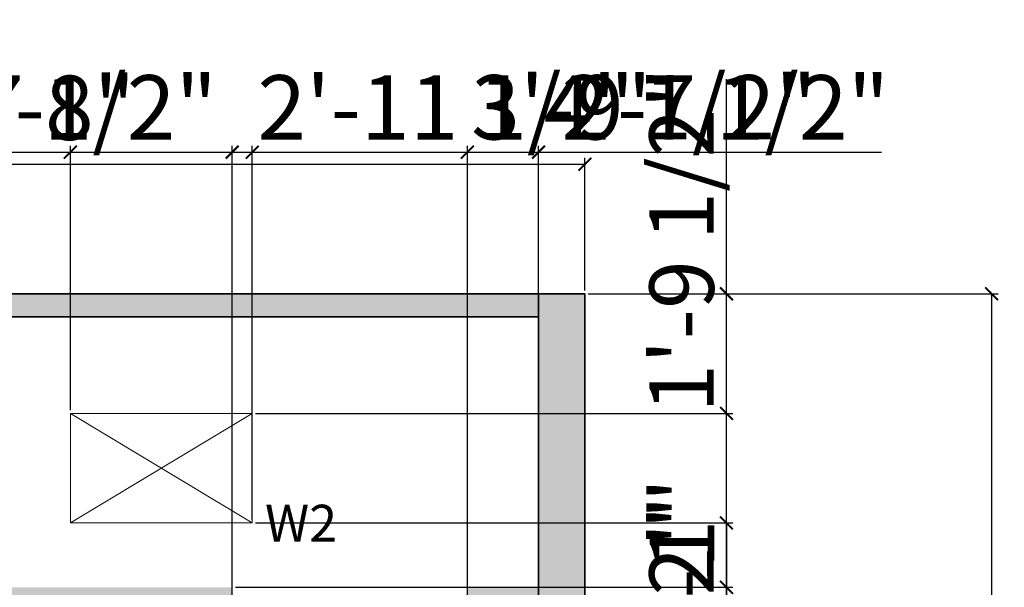
# Model space of a CAD drawing. Units: inches. Extents: x 1763 to 2368, y 1500 to 2097.
# Tile 23 of 24: x 2079 to 2271, y 1986 to 2097. Entities that reach past the tile are written whole.
import ezdxf

# ---------------------------------------------------------------- set-up
doc = ezdxf.new("R2010")
doc.units = ezdxf.units.IN
for name, color, linetype, lineweight in [('A-ANNO-DIMS', 2, 'Continuous', 18), ('A-ANNO-TEXT', 7, 'Continuous', 18), ('A-WALL', 7, 'Continuous', 35), ('A-WALL-PATT', 7, 'Continuous', 13), ('C-SITE-FIXT', 8, 'Continuous', 18)]:
    doc.layers.add(name, color=color, linetype=linetype, lineweight=lineweight)
doc.styles.get("Standard").update_dxf_attribs({"font": 'arial.ttf'})
doc.dimstyles.new('ISO-25', dxfattribs={"dimtxt": 12.5, "dimasz": 2.5, "dimexe": 1.25, "dimexo": 0.625, "dimtad": 1, "dimdec": 0, "dimlunit": 4, "dimtxsty": 'Standard', "dimblk": 'ARCHTICK', "dimcen": 2.5, "dimclrd": 3, "dimclrt": 4, "dimadec": 0, "dimazin": 0, "dimtfac": 1, "dimtdec": 0, "dimtmove": 0, "dimatfit": 3, "dimfxl": 1, "dimarcsym": 0})

# ---------------------------------------------------------------- blocks, each defined once
blk = doc.blocks.new('_ArchTick')
at = {"color": 0, "linetype": 'ByBlock', "const_width": 0.15}
blk.add_lwpolyline([(-0.5, -0.5), (0.5, 0.5)], dxfattribs=at)
blk = doc.blocks.new('*D21')
at = {"layer": 'A-ANNO-DIMS', "color": 0, "lineweight": -2, "transparency": 16777216}
for p, q in [((1829.09, 2043.9), (1829.09, 2069.68)), ((1829.09, 2068.43), (2189.09, 2068.43)), ((2189.09, 2043.9), (2189.09, 2069.68))]:
    blk.add_line(p, q, dxfattribs=at)
at = {"layer": 'Defpoints', "color": 0, "transparency": 16777216}
for p in [(2189.09, 2068.43), (1829.09, 2043.27), (2189.09, 2043.27)]:
    blk.add_point(p, dxfattribs=at)
at = {"layer": 'A-ANNO-DIMS', "color": 0, "lineweight": -2, "transparency": 16777216, "xscale": 2.5, "yscale": 2.5, "zscale": 2.5, "rotation": 180}
blk.add_blockref('_ArchTick', (1829.09, 2068.43), dxfattribs=at)
at = {"layer": 'A-ANNO-DIMS', "color": 0, "lineweight": -2, "transparency": 16777216, "xscale": 2.5, "yscale": 2.5, "zscale": 2.5}
blk.add_blockref('_ArchTick', (2189.09, 2068.43), dxfattribs=at)
at = {"layer": 'A-ANNO-DIMS', "color": 0, "transparency": 16777216, "insert": (2009.09, 2075.45), "char_height": 12.5, "attachment_point": 5}
blk.add_mtext("30'", dxfattribs=at)
blk = doc.blocks.new('*D22')
at = {"layer": 'A-ANNO-DIMS', "color": 0, "lineweight": -2, "transparency": 16777216}
for p, q in [((2189.72, 2043.27), (2269.32, 2043.27)), ((2268.07, 2043.27), (2268.07, 1563.27)), ((2189.72, 1563.27), (2269.32, 1563.27))]:
    blk.add_line(p, q, dxfattribs=at)
at = {"layer": 'Defpoints', "color": 0, "transparency": 16777216}
for p in [(2189.09, 2043.27), (2189.09, 1563.27), (2268.07, 1563.27)]:
    blk.add_point(p, dxfattribs=at)
at = {"layer": 'A-ANNO-DIMS', "color": 0, "lineweight": -2, "transparency": 16777216, "xscale": 2.5, "yscale": 2.5, "zscale": 2.5}
for p, rotation in [((2268.07, 2043.27), 90), ((2268.07, 1563.27), 270)]:
    blk.add_blockref('_ArchTick', p, dxfattribs=dict(at, rotation=rotation))
at = {"layer": 'A-ANNO-DIMS', "color": 0, "transparency": 16777216, "insert": (2261.06, 1803.27), "char_height": 12.5, "attachment_point": 5, "rotation": 90}
blk.add_mtext("40'", dxfattribs=at)
blk = doc.blocks.new('*D23')
at = {"layer": 'A-ANNO-DIMS', "color": 0, "lineweight": -2, "transparency": 16777216}
for p, q in [((2089.48, 1949.98), (2089.48, 1963.99)), ((2178.7, 1949.98), (2178.7, 1963.99))]:
    blk.add_line(p, q, dxfattribs=at)
at = {"layer": 'A-ANNO-DIMS', "color": 3, "lineweight": -2, "transparency": 16777216}
for p, q in [((2089.48, 1962.74), (2178.7, 1962.74)), ((2178.7, 1962.74), (2367.73, 1962.74))]:
    blk.add_line(p, q, dxfattribs=at)
at = {"layer": 'Defpoints', "color": 0, "transparency": 16777216}
for p in [(2178.7, 1962.74), (2089.48, 1949.35), (2178.7, 1949.35)]:
    blk.add_point(p, dxfattribs=at)
at = {"layer": 'A-ANNO-DIMS', "color": 3, "lineweight": -2, "transparency": 16777216, "xscale": 2.5, "yscale": 2.5, "zscale": 2.5, "rotation": 180}
blk.add_blockref('_ArchTick', (2089.48, 1962.74), dxfattribs=at)
at = {"layer": 'A-ANNO-DIMS', "color": 3, "lineweight": -2, "transparency": 16777216, "xscale": 2.5, "yscale": 2.5, "zscale": 2.5}
blk.add_blockref('_ArchTick', (2178.7, 1962.74), dxfattribs=at)
at = {"layer": 'A-ANNO-DIMS', "color": 4, "transparency": 16777216, "insert": (2274.46, 1969.83), "char_height": 12.5, "attachment_point": 5}
blk.add_mtext('BED GROUP 7\'-5" TYP.', dxfattribs=at)
blk = doc.blocks.new('*D55')
at = {"layer": 'A-ANNO-DIMS', "color": 3, "lineweight": -2, "transparency": 16777216}
for p, q in [((2216.59, 1934.11), (2216.59, 2000.72)), ((2216.59, 1885.52), (2216.59, 1934.11))]:
    blk.add_line(p, q, dxfattribs=at)
at = {"layer": 'A-ANNO-DIMS', "color": 0, "lineweight": -2, "transparency": 16777216}
for p, q in [((2189.72, 1934.11), (2217.84, 1934.11)), ((2189.72, 1885.52), (2217.84, 1885.52))]:
    blk.add_line(p, q, dxfattribs=at)
at = {"layer": 'Defpoints', "color": 0, "transparency": 16777216}
for p in [(2189.09, 1934.11), (2216.59, 1934.11), (2189.09, 1885.52)]:
    blk.add_point(p, dxfattribs=at)
at = {"layer": 'A-ANNO-DIMS', "color": 3, "lineweight": -2, "transparency": 16777216, "xscale": 2.5, "yscale": 2.5, "zscale": 2.5}
for p, rotation in [((2216.59, 1934.11), 90), ((2216.59, 1885.52), 270)]:
    blk.add_blockref('_ArchTick', p, dxfattribs=dict(at, rotation=rotation))
at = {"layer": 'A-ANNO-DIMS', "color": 4, "transparency": 16777216, "insert": (2209.5, 1968.66), "char_height": 12.5, "attachment_point": 5, "rotation": 90}
blk.add_mtext('4\'-0 1/2"', dxfattribs=at)
blk = doc.blocks.new('*D56')
at = {"layer": 'A-ANNO-DIMS', "color": 0, "lineweight": -2, "transparency": 16777216}
for p, q in [((2189.72, 2043.27), (2217.84, 2043.27)), ((2189.72, 1934.11), (2217.84, 1934.11))]:
    blk.add_line(p, q, dxfattribs=at)
at = {"layer": 'A-ANNO-DIMS', "color": 3, "lineweight": -2, "transparency": 16777216}
blk.add_line((2216.59, 1934.11), (2216.59, 2043.27), dxfattribs=at)
at = {"layer": 'Defpoints', "color": 0, "transparency": 16777216}
for p in [(2189.09, 2043.27), (2216.59, 2043.27), (2189.09, 1934.11)]:
    blk.add_point(p, dxfattribs=at)
at = {"layer": 'A-ANNO-DIMS', "color": 3, "lineweight": -2, "transparency": 16777216, "xscale": 2.5, "yscale": 2.5, "zscale": 2.5}
for p, rotation in [((2216.59, 2043.27), 90), ((2216.59, 1934.11), 270)]:
    blk.add_blockref('_ArchTick', p, dxfattribs=dict(at, rotation=rotation))
at = {"layer": 'A-ANNO-DIMS', "color": 4, "transparency": 16777216, "insert": (2209.58, 1988.69), "char_height": 12.5, "attachment_point": 5, "rotation": 90}
blk.add_mtext('9\'-1"', dxfattribs=at)
blk = doc.blocks.new('*D63')
at = {"layer": 'A-ANNO-DIMS', "color": 0, "lineweight": -2, "transparency": 16777216}
for p, q in [((2120.61, 1981.9), (2120.61, 2072.02)), ((2166.28, 1981.9), (2166.28, 2072.02))]:
    blk.add_line(p, q, dxfattribs=at)
at = {"layer": 'A-ANNO-DIMS', "color": 3, "lineweight": -2, "transparency": 16777216}
for p, q in [((2120.61, 2070.77), (2166.28, 2070.77)), ((2166.28, 2070.77), (2232.38, 2070.77))]:
    blk.add_line(p, q, dxfattribs=at)
at = {"layer": 'Defpoints', "color": 0, "transparency": 16777216}
for p in [(2166.28, 2070.77), (2120.61, 1981.27), (2166.28, 1981.27)]:
    blk.add_point(p, dxfattribs=at)
at = {"layer": 'A-ANNO-DIMS', "color": 3, "lineweight": -2, "transparency": 16777216, "xscale": 2.5, "yscale": 2.5, "zscale": 2.5, "rotation": 180}
blk.add_blockref('_ArchTick', (2120.61, 2070.77), dxfattribs=at)
at = {"layer": 'A-ANNO-DIMS', "color": 3, "lineweight": -2, "transparency": 16777216, "xscale": 2.5, "yscale": 2.5, "zscale": 2.5}
blk.add_blockref('_ArchTick', (2166.28, 2070.77), dxfattribs=at)
at = {"layer": 'A-ANNO-DIMS', "color": 4, "transparency": 16777216, "insert": (2200.58, 2077.87), "char_height": 12.5, "attachment_point": 5}
blk.add_mtext('3\'-9 1/2"', dxfattribs=at)
blk = doc.blocks.new('*D72')
at = {"layer": 'A-ANNO-DIMS', "color": 0, "lineweight": -2, "transparency": 16777216}
for p, q in [((2018.09, 1885.9), (2018.09, 2072.02)), ((2049.74, 1885.9), (2049.74, 2072.02))]:
    blk.add_line(p, q, dxfattribs=at)
at = {"layer": 'A-ANNO-DIMS', "color": 3, "lineweight": -2, "transparency": 16777216}
for p, q in [((2018.09, 2070.77), (2049.74, 2070.77)), ((2049.74, 2070.77), (2116.06, 2070.77))]:
    blk.add_line(p, q, dxfattribs=at)
at = {"layer": 'Defpoints', "color": 0, "transparency": 16777216}
for p in [(2049.74, 2070.77), (2018.09, 1885.27), (2049.74, 1885.27)]:
    blk.add_point(p, dxfattribs=at)
at = {"layer": 'A-ANNO-DIMS', "color": 3, "lineweight": -2, "transparency": 16777216, "xscale": 2.5, "yscale": 2.5, "zscale": 2.5, "rotation": 180}
blk.add_blockref('_ArchTick', (2018.09, 2070.77), dxfattribs=at)
at = {"layer": 'A-ANNO-DIMS', "color": 3, "lineweight": -2, "transparency": 16777216, "xscale": 2.5, "yscale": 2.5, "zscale": 2.5}
blk.add_blockref('_ArchTick', (2049.74, 2070.77), dxfattribs=at)
at = {"layer": 'A-ANNO-DIMS', "color": 4, "transparency": 16777216, "insert": (2084.15, 2077.86), "char_height": 12.5, "attachment_point": 5}
blk.add_mtext('2\'-7 1/2"', dxfattribs=at)
blk = doc.blocks.new('*D76')
at = {"layer": 'A-ANNO-DIMS', "color": 0, "lineweight": -2, "transparency": 16777216}
for p, q in [((2031.02, 1986.9), (2031.02, 2072.02)), ((2063.14, 1986.9), (2063.14, 2072.02))]:
    blk.add_line(p, q, dxfattribs=at)
at = {"layer": 'A-ANNO-DIMS', "color": 3, "lineweight": -2, "transparency": 16777216}
for p, q in [((2031.02, 2070.77), (2063.14, 2070.77)), ((2063.14, 2070.77), (2100.33, 2070.77))]:
    blk.add_line(p, q, dxfattribs=at)
at = {"layer": 'Defpoints', "color": 0, "transparency": 16777216}
for p in [(2063.14, 2070.77), (2031.02, 1986.27), (2063.14, 1986.27)]:
    blk.add_point(p, dxfattribs=at)
at = {"layer": 'A-ANNO-DIMS', "color": 3, "lineweight": -2, "transparency": 16777216, "xscale": 2.5, "yscale": 2.5, "zscale": 2.5, "rotation": 180}
blk.add_blockref('_ArchTick', (2031.02, 2070.77), dxfattribs=at)
at = {"layer": 'A-ANNO-DIMS', "color": 3, "lineweight": -2, "transparency": 16777216, "xscale": 2.5, "yscale": 2.5, "zscale": 2.5}
blk.add_blockref('_ArchTick', (2063.14, 2070.77), dxfattribs=at)
at = {"layer": 'A-ANNO-DIMS', "color": 4, "transparency": 16777216, "insert": (2082.99, 2077.78), "char_height": 12.5, "attachment_point": 5}
blk.add_mtext('2\'-8"', dxfattribs=at)
blk = doc.blocks.new('*D92')
at = {"layer": 'A-ANNO-DIMS', "color": 0, "lineweight": -2, "transparency": 16777216}
for p, q in [((2089.21, 2020.67), (2089.21, 2072.02)), ((2124.53, 2020.67), (2124.53, 2072.02))]:
    blk.add_line(p, q, dxfattribs=at)
at = {"layer": 'A-ANNO-DIMS', "color": 3, "lineweight": -2, "transparency": 16777216}
for p, q in [((2089.21, 2070.77), (2124.53, 2070.77)), ((2124.53, 2070.77), (2200.56, 2070.77))]:
    blk.add_line(p, q, dxfattribs=at)
at = {"layer": 'Defpoints', "color": 0, "transparency": 16777216}
for p in [(2124.53, 2070.77), (2089.21, 2020.04), (2124.53, 2020.04)]:
    blk.add_point(p, dxfattribs=at)
at = {"layer": 'A-ANNO-DIMS', "color": 3, "lineweight": -2, "transparency": 16777216, "xscale": 2.5, "yscale": 2.5, "zscale": 2.5, "rotation": 180}
blk.add_blockref('_ArchTick', (2089.21, 2070.77), dxfattribs=at)
at = {"layer": 'A-ANNO-DIMS', "color": 3, "lineweight": -2, "transparency": 16777216, "xscale": 2.5, "yscale": 2.5, "zscale": 2.5}
blk.add_blockref('_ArchTick', (2124.53, 2070.77), dxfattribs=at)
at = {"layer": 'A-ANNO-DIMS', "color": 4, "transparency": 16777216, "insert": (2163.8, 2077.86), "char_height": 12.5, "attachment_point": 5}
blk.add_mtext('2\'-11 1/2"', dxfattribs=at)
blk = doc.blocks.new('*D93')
at = {"layer": 'A-ANNO-DIMS', "color": 0, "lineweight": -2, "transparency": 16777216}
for p, q in [((2124.53, 1999.39), (2124.53, 2072.02)), ((2180.09, 1986.9), (2180.09, 2072.02))]:
    blk.add_line(p, q, dxfattribs=at)
at = {"layer": 'A-ANNO-DIMS', "color": 3, "lineweight": -2, "transparency": 16777216}
for p, q in [((2124.53, 2070.77), (2180.09, 2070.77)), ((2180.09, 2070.77), (2246.7, 2070.77))]:
    blk.add_line(p, q, dxfattribs=at)
at = {"layer": 'Defpoints', "color": 0, "transparency": 16777216}
for p in [(2180.09, 2070.77), (2124.53, 1998.77), (2180.09, 1986.27)]:
    blk.add_point(p, dxfattribs=at)
at = {"layer": 'A-ANNO-DIMS', "color": 3, "lineweight": -2, "transparency": 16777216, "xscale": 2.5, "yscale": 2.5, "zscale": 2.5, "rotation": 180}
blk.add_blockref('_ArchTick', (2124.53, 2070.77), dxfattribs=at)
at = {"layer": 'A-ANNO-DIMS', "color": 3, "lineweight": -2, "transparency": 16777216, "xscale": 2.5, "yscale": 2.5, "zscale": 2.5}
blk.add_blockref('_ArchTick', (2180.09, 2070.77), dxfattribs=at)
at = {"layer": 'A-ANNO-DIMS', "color": 4, "transparency": 16777216, "insert": (2214.65, 2077.86), "char_height": 12.5, "attachment_point": 5}
blk.add_mtext('4\'-7 1/2"', dxfattribs=at)
blk = doc.blocks.new('*D94')
at = {"layer": 'A-ANNO-DIMS', "color": 3, "lineweight": -2, "transparency": 16777216}
for p, q in [((2216.59, 2020.04), (2216.59, 2084.97)), ((2216.59, 1998.77), (2216.59, 2020.04))]:
    blk.add_line(p, q, dxfattribs=at)
at = {"layer": 'A-ANNO-DIMS', "color": 0, "lineweight": -2, "transparency": 16777216}
for p, q in [((2125.16, 2020.04), (2217.84, 2020.04)), ((2125.16, 1998.77), (2217.84, 1998.77))]:
    blk.add_line(p, q, dxfattribs=at)
at = {"layer": 'Defpoints', "color": 0, "transparency": 16777216}
for p in [(2124.53, 2020.04), (2216.59, 2020.04), (2124.53, 1998.77)]:
    blk.add_point(p, dxfattribs=at)
at = {"layer": 'A-ANNO-DIMS', "color": 3, "lineweight": -2, "transparency": 16777216, "xscale": 2.5, "yscale": 2.5, "zscale": 2.5}
for p, rotation in [((2216.59, 2020.04), 90), ((2216.59, 1998.77), 270)]:
    blk.add_blockref('_ArchTick', p, dxfattribs=dict(at, rotation=rotation))
at = {"layer": 'A-ANNO-DIMS', "color": 4, "transparency": 16777216, "insert": (2209.5, 2053.76), "char_height": 12.5, "attachment_point": 5, "rotation": 90}
blk.add_mtext('1\'-9 1/2"', dxfattribs=at)
blk = doc.blocks.new('*D95')
at = {"layer": 'A-ANNO-DIMS', "color": 0, "lineweight": -2, "transparency": 16777216}
for p, q in [((2125.16, 1998.77), (2217.84, 1998.77)), ((2121.24, 1986.27), (2217.84, 1986.27))]:
    blk.add_line(p, q, dxfattribs=at)
at = {"layer": 'A-ANNO-DIMS', "color": 3, "lineweight": -2, "transparency": 16777216}
for p, q in [((2216.59, 1998.77), (2216.59, 1986.27)), ((2216.59, 1986.27), (2216.59, 1921.34))]:
    blk.add_line(p, q, dxfattribs=at)
at = {"layer": 'Defpoints', "color": 0, "transparency": 16777216}
for p in [(2124.53, 1998.77), (2120.61, 1986.27), (2216.59, 1986.27)]:
    blk.add_point(p, dxfattribs=at)
at = {"layer": 'A-ANNO-DIMS', "color": 3, "lineweight": -2, "transparency": 16777216, "xscale": 2.5, "yscale": 2.5, "zscale": 2.5}
for p, rotation in [((2216.59, 1998.77), 90), ((2216.59, 1986.27), 270)]:
    blk.add_blockref('_ArchTick', p, dxfattribs=dict(at, rotation=rotation))
at = {"layer": 'A-ANNO-DIMS', "color": 4, "transparency": 16777216, "insert": (2209.5, 1952.56), "char_height": 12.5, "attachment_point": 5, "rotation": 90}
blk.add_mtext('1\'-0 1/2"', dxfattribs=at)

msp = doc.modelspace()

# ---------------------------------------------------------------- hatches: boundary and pattern name
at = {"layer": 'A-WALL-PATT'}
h = msp.add_hatch(color=256, dxfattribs=at)
h.dxf.hatch_style = 1
h.paths.add_polyline_path([(1838.09, 2034.27), (1838.09, 2043.27), (1829.09, 2043.27), (1829.09, 1953.39), (1838.09, 1953.39)])
h.paths.add_polyline_path([(1838.09, 1913.1), (1829.09, 1913.1), (1829.09, 1862.2), (1838.09, 1862.2)])
h.paths.add_polyline_path([(1838.09, 1825.59), (1829.09, 1825.59), (1829.09, 1738.64), (1838.09, 1738.64)])
h.paths.add_polyline_path([(1895.59, 1885.27), (1838.09, 1885.27), (1838.09, 1880.27), (1895.59, 1880.27)])
h.paths.add_polyline_path([(1857.39, 1784.27), (1838.09, 1784.27), (1838.09, 1779.27), (1857.39, 1779.27)])
h.paths.add_polyline_path([(1958.09, 1981.27), (1971.46, 1981.27), (1971.46, 1986.27), (1968.57, 1986.27), (1958.09, 1986.27), (1953.09, 1986.27), (1927.39, 1986.27), (1927.39, 1981.27), (1953.09, 1981.27), (1953.09, 1885.27), (1932.01, 1885.27), (1932.01, 1880.27), (1959.13, 1880.27), (1959.13, 1883.74), (1959.13, 1885.27), (1958.09, 1885.27)])
h.paths.add_polyline_path([(2018.09, 1981.27), (2031.02, 1981.27), (2031.02, 1986.27), (2018.09, 1986.27), (2013.09, 1986.27), (2001.23, 1986.27), (2001.23, 1981.27), (2013.09, 1981.27), (2013.09, 1885.27), (1982.18, 1885.27, -0.016629), (1982.23, 1883.74), (1982.23, 1880.27), (2049.69, 1880.27), (2049.69, 1883.74, -0.016629), (2049.74, 1885.27), (2018.09, 1885.27)])
h.paths.add_polyline_path([(2083.09, 1981.27), (2120.61, 1981.27), (2120.61, 1986.27), (2083.09, 1986.27), (2078.09, 1986.27), (2063.14, 1986.27), (2063.14, 1981.27), (2078.09, 1981.27), (2078.09, 1885.27), (2072.78, 1885.27), (2072.78, 1883.74), (2072.78, 1880.27), (2078.09, 1880.27), (2078.09, 1866.87), (2081.56, 1866.87, -0.016629), (2083.09, 1866.82)])
h.paths.add_polyline_path([(1871.68, 1635.27), (1838.09, 1635.27), (1838.09, 1626.27), (1871.68, 1626.27)], flags=17)
h.paths.add_polyline_path([(2100.58, 1688.27), (2060.09, 1688.27), (2060.09, 1679.27), (2100.58, 1679.27)], flags=17)
h.paths.add_polyline_path([(2180.09, 1688.27), (2148.74, 1688.27), (2148.74, 1679.27), (2180.09, 1679.27)], flags=17)
h.paths.add_polyline_path([(2189.09, 1746.22), (2180.09, 1746.22), (2180.09, 1743.42), (2180.12, 1743.42), (2180.12, 1726.72), (2180.09, 1572.27), (2034.91, 1572.27), (2034.91, 1565.6), (2034.91, 1563.27), (2189.09, 1563.27)])
h.paths.add_polyline_path([(2060.09, 1802.35, -0.016629), (2058.56, 1802.3), (2055.09, 1802.3), (2055.09, 1635.27), (2042.48, 1635.27), (2042.48, 1629.74), (2042.48, 1626.27), (2055.09, 1626.27), (2055.09, 1599.27), (2040.27, 1599.27), (2040.27, 1590.27), (2060.09, 1590.27)])
h.paths.add_polyline_path([(2019.39, 1629.74, -0.060569), (2020.06, 1635.27), (1995.09, 1635.27), (1990.09, 1635.27), (1927.07, 1635.27), (1927.07, 1626.27), (1990.09, 1626.27), (1990.09, 1590.27), (1995.09, 1590.27), (2005.2, 1590.27), (2005.2, 1599.27), (1995.09, 1599.27), (1995.09, 1626.27), (2019.39, 1626.27)])
edge = h.paths.add_edge_path()
edge.add_line((2180.09, 1837.27), (2167.2, 1837.27))
edge.add_spline(control_points=[(2167.2, 1837.27), (2167.19, 1837.27), (2167.18, 1837.27), (2167.18, 1837.27)], knot_values=[168.955493, 168.955493, 168.955493, 168.955493, 169.065871, 169.065871, 169.065871, 169.065871], degree=3, periodic=0)
edge.add_spline(control_points=[(2167.18, 1837.27), (2166.56, 1837.38), (2166.33, 1846.16), (2165.71, 1846.24)], knot_values=[159.864705, 159.864705, 159.864705, 159.864705, 168.955493, 168.955493, 168.955493, 168.955493], degree=3, periodic=0)
edge.add_line((2167.12, 1837.27), (2163.16, 1837.27))
edge.add_spline(control_points=[(2163.16, 1837.27), (2163.16, 1837.27), (2163.16, 1837.27), (2163.15, 1837.27)], knot_values=[150.537172, 150.537172, 150.537172, 150.537172, 150.553797, 150.553797, 150.553797, 150.553797], degree=3, periodic=0)
edge.add_spline(control_points=[(2163.15, 1837.27), (2162.29, 1837.29), (2161.59, 1846.23), (2160.88, 1846.24)], knot_values=[141.293426, 141.293426, 141.293426, 141.293426, 150.537172, 150.537172, 150.537172, 150.537172], degree=3, periodic=0)
edge.add_line((2163.08, 1837.27), (2158.7, 1837.27))
edge.add_spline(control_points=[(2158.7, 1837.27), (2158.7, 1837.27), (2158.7, 1837.27), (2158.7, 1837.27)], knot_values=[132.033544, 132.033544, 132.033544, 132.033544, 132.049151, 132.049151, 132.049151, 132.049151], degree=3, periodic=0)
edge.add_spline(control_points=[(2158.7, 1837.27), (2157.97, 1837.29), (2157.26, 1846.23), (2156.39, 1846.24)], knot_values=[122.786021, 122.786021, 122.786021, 122.786021, 132.033544, 132.033544, 132.033544, 132.033544], degree=3, periodic=0)
edge.add_line((2158.63, 1837.27), (2153.84, 1837.27))
edge.add_spline(control_points=[(2153.84, 1837.27), (2153.83, 1837.27), (2153.82, 1837.27), (2153.82, 1837.27)], knot_values=[113.451585, 113.451585, 113.451585, 113.451585, 113.562103, 113.562103, 113.562103, 113.562103], degree=3, periodic=0)
edge.add_spline(control_points=[(2153.82, 1837.27), (2153.17, 1837.38), (2152.88, 1846.19), (2152.4, 1846.24)], knot_values=[0, 0, 0, 0, 9.081854, 9.081854, 9.081854, 9.081854], degree=3, periodic=0)
edge.add_line((2153.76, 1837.27), (2150.39, 1837.27))
edge.add_spline(control_points=[(2150.39, 1837.27), (2150.38, 1837.27), (2150.37, 1837.27), (2150.36, 1837.27)], knot_values=[95.069382, 95.069382, 95.069382, 95.069382, 95.17519, 95.17519, 95.17519, 95.17519], degree=3, periodic=0)
edge.add_spline(control_points=[(2150.36, 1837.27), (2149.49, 1837.37), (2148.42, 1846.19), (2147.59, 1846.24)], knot_values=[85.824599, 85.824599, 85.824599, 85.824599, 95.069382, 95.069382, 95.069382, 95.069382], degree=3, periodic=0)
edge.add_line((2150.29, 1837.27), (2145.43, 1837.27))
edge.add_spline(control_points=[(2145.43, 1837.27), (2145.43, 1837.27), (2145.42, 1837.27), (2145.42, 1837.27)], knot_values=[76.505559, 76.505559, 76.505559, 76.505559, 76.547811, 76.547811, 76.547811, 76.547811], degree=3, periodic=0)
edge.add_spline(control_points=[(2145.42, 1837.27), (2144.68, 1837.31), (2143.8, 1846.19), (2142.95, 1846.24)], knot_values=[67.23945, 67.23945, 67.23945, 67.23945, 76.505559, 76.505559, 76.505559, 76.505559], degree=3, periodic=0)
edge.add_line((2145.35, 1837.27), (2134.57, 1837.27))
edge.add_spline(control_points=[(2134.57, 1837.27), (2134.57, 1837.27), (2134.56, 1837.27), (2134.56, 1837.27)], knot_values=[39.001463, 39.001463, 39.001463, 39.001463, 39.045107, 39.045107, 39.045107, 39.045107], degree=3, periodic=0)
edge.add_spline(control_points=[(2134.56, 1837.27), (2133.87, 1837.31), (2133.4, 1845.85), (2132.33, 1846.24)], knot_values=[29.79778, 29.79778, 29.79778, 29.79778, 39.001463, 39.001463, 39.001463, 39.001463], degree=3, periodic=0)
edge.add_line((2134.5, 1837.27), (2128.08, 1837.27))
edge.add_spline(control_points=[(2128.08, 1837.27), (2128.03, 1837.26), (2127.98, 1837.26), (2127.93, 1837.27)], knot_values=[19.482067, 19.482067, 19.482067, 19.482067, 19.869396, 19.869396, 19.869396, 19.869396], degree=3, periodic=0)
edge.add_spline(control_points=[(2125.01, 1846.24), (2126.16, 1844.66), (2126.82, 1837.57), (2127.93, 1837.27)], knot_values=[10.389805, 10.389805, 10.389805, 10.389805, 19.482067, 19.482067, 19.482067, 19.482067], degree=3, periodic=0)
edge.add_line((2127.93, 1837.27), (2083.09, 1837.27))
edge.add_line((2083.09, 1837.27), (2083.09, 1843.77))
edge.add_line((2083.09, 1843.77), (2081.56, 1843.77))
edge.add_line((2081.56, 1843.77), (2078.09, 1843.77))
edge.add_line((2078.09, 1843.77), (2078.09, 1837.27))
edge.add_line((2078.09, 1837.27), (2055.09, 1837.27))
edge.add_line((2055.09, 1837.27), (2055.09, 1825.4))
edge.add_line((2055.09, 1825.4), (2058.56, 1825.4))
edge.add_line((2058.56, 1825.4), (2060.09, 1825.4))
edge.add_line((2060.09, 1825.4), (2060.09, 1832.27))
edge.add_line((2060.09, 1832.27), (2122.44, 1832.27))
edge.add_spline(control_points=[(2122.44, 1832.27), (2122.73, 1832.58), (2123.01, 1832.62), (2123.28, 1832.27)], knot_values=[5.972033, 5.972033, 5.972033, 5.972033, 8.057258, 8.057258, 8.057258, 8.057258], degree=3, periodic=0)
edge.add_line((2123.28, 1832.27), (2137.95, 1832.27))
edge.add_spline(control_points=[(2137.95, 1832.27), (2137.96, 1832.27), (2137.97, 1832.27), (2137.98, 1832.27)], knot_values=[53.926862, 53.926862, 53.926862, 53.926862, 54.030075, 54.030075, 54.030075, 54.030075], degree=3, periodic=0)
edge.add_spline(control_points=[(2139.72, 1825.02), (2139.28, 1825.06), (2138.67, 1832.18), (2137.98, 1832.27)], knot_values=[54.030075, 54.030075, 54.030075, 54.030075, 61.445194, 61.445194, 61.445194, 61.445194], degree=3, periodic=0)
edge.add_line((2138.05, 1832.27), (2140.96, 1832.27))
edge.add_spline(control_points=[(2140.96, 1832.27), (2140.97, 1832.27), (2140.98, 1832.27), (2140.99, 1832.27)], knot_values=[68.854182, 68.854182, 68.854182, 68.854182, 68.971237, 68.971237, 68.971237, 68.971237], degree=3, periodic=0)
edge.add_spline(control_points=[(2143.19, 1825.02), (2142.44, 1825.07), (2141.56, 1832.16), (2140.99, 1832.27)], knot_values=[68.971237, 68.971237, 68.971237, 68.971237, 76.444911, 76.444911, 76.444911, 76.444911], degree=3, periodic=0)
edge.add_line((2141.04, 1832.27), (2145.43, 1832.27))
edge.add_spline(control_points=[(2145.43, 1832.27), (2145.44, 1832.27), (2145.45, 1832.27), (2145.46, 1832.27)], knot_values=[84.039047, 84.039047, 84.039047, 84.039047, 84.124041, 84.124041, 84.124041, 84.124041], degree=3, periodic=0)
edge.add_spline(control_points=[(2148.11, 1825.02), (2147.34, 1825.02), (2146.3, 1832.19), (2145.46, 1832.27)], knot_values=[84.124041, 84.124041, 84.124041, 84.124041, 91.773891, 91.773891, 91.773891, 91.773891], degree=3, periodic=0)
edge.add_line((2145.54, 1832.27), (2150.39, 1832.27))
edge.add_spline(control_points=[(2150.39, 1832.27), (2150.42, 1832.28), (2150.45, 1832.28), (2150.47, 1832.27)], knot_values=[99.381577, 99.381577, 99.381577, 99.381577, 99.573457, 99.573457, 99.573457, 99.573457], degree=3, periodic=0)
edge.add_spline(control_points=[(2153.97, 1825.02), (2153.09, 1825.28), (2151.53, 1832.1), (2150.47, 1832.27)], knot_values=[99.573457, 99.573457, 99.573457, 99.573457, 107.218357, 107.218357, 107.218357, 107.218357], degree=3, periodic=0)
edge.add_line((2150.57, 1832.27), (2155.6, 1832.27))
edge.add_spline(control_points=[(2155.6, 1832.27), (2155.6, 1832.27), (2155.61, 1832.27), (2155.62, 1832.27)], knot_values=[114.933058, 114.933058, 114.933058, 114.933058, 115.013624, 115.013624, 115.013624, 115.013624], degree=3, periodic=0)
edge.add_spline(control_points=[(2158.28, 1825.02), (2157.4, 1825.07), (2156.25, 1832.2), (2155.62, 1832.27)], knot_values=[115.013624, 115.013624, 115.013624, 115.013624, 122.616269, 122.616269, 122.616269, 122.616269], degree=3, periodic=0)
edge.add_line((2155.68, 1832.27), (2165.19, 1832.27))
edge.add_spline(control_points=[(2165.19, 1832.27), (2165.2, 1832.27), (2165.2, 1832.27), (2165.2, 1832.27)], knot_values=[145.488477, 145.488477, 145.488477, 145.488477, 145.516379, 145.516379, 145.516379, 145.516379], degree=3, periodic=0)
edge.add_spline(control_points=[(2167.45, 1825.02), (2166.96, 1825.02), (2166.06, 1832.25), (2165.2, 1832.27)], knot_values=[145.516379, 145.516379, 145.516379, 145.516379, 153.105469, 153.105469, 153.105469, 153.105469], degree=3, periodic=0)
edge.add_line((2165.29, 1832.27), (2168.93, 1832.27))
edge.add_spline(control_points=[(2168.93, 1832.27), (2168.98, 1832.29), (2169.04, 1832.29), (2169.1, 1832.27)], knot_values=[160.517439, 160.517439, 160.517439, 160.517439, 160.939723, 160.939723, 160.939723, 160.939723], degree=3, periodic=0)
edge.add_spline(control_points=[(2171.09, 1828.64), (2170.35, 1830.37), (2169.62, 1832.09), (2169.1, 1832.27)], knot_values=[160.939723, 160.939723, 160.939723, 160.939723, 164.738835, 164.738835, 164.738835, 164.738835], degree=3, periodic=0)
edge.add_line((2169.1, 1832.27), (2180.09, 1832.27))
edge.add_line((2180.09, 1832.27), (2180.09, 1837.27))
h.paths.add_polyline_path([(2189.09, 1885.52), (2180.09, 1885.52), (2180.09, 1813.32), (2180.12, 1813.32), (2180.12, 1796.62), (2180.12, 1795.26), (2189.09, 1795.26)])
h.paths.add_polyline_path([(2180.09, 1986.27), (2166.28, 1986.27), (2166.28, 1981.27), (2180.09, 1981.27)])
h.paths.add_polyline_path([(2189.09, 2043.27), (2180.09, 2043.27), (2180.09, 2034.27), (2180.09, 1934.11), (2189.09, 1934.11)])
h.paths.add_polyline_path([(1838.09, 1681.59), (1829.09, 1681.59), (1829.09, 1563.27), (2003.86, 1563.27), (2003.86, 1565.6), (2003.86, 1572.27), (1838.09, 1572.27)])
h = msp.add_hatch(color=256, dxfattribs=at)
h.dxf.hatch_style = 1
h.paths.add_polyline_path([(2180.09, 2043.27), (1838.09, 2043.27), (1838.09, 2038.83), (2180.09, 2038.83)])

# ---------------------------------------------------------------- linework, layer by layer
at = {"layer": 'A-WALL'}
for p, q in [((1838.09, 2043.27), (2180.09, 2043.27)), ((2180.09, 2034.27), (2180.09, 2043.27)), ((1838.09, 2038.83), (2180.09, 2038.83)), ((2180.09, 2034.27), (2180.09, 1572.27))]:
    msp.add_line(p, q, dxfattribs=at)
msp.add_lwpolyline([(2003.86, 1563.27), (1829.09, 1563.27), (1829.09, 2043.27), (2189.09, 2043.27), (2189.09, 1563.27), (2034.91, 1563.27)], dxfattribs=at)
at = {"layer": 'C-SITE-FIXT'}
for p, q in [((2089.21, 2020.04), (2124.53, 1998.77)), ((2124.53, 2020.04), (2089.21, 1998.77))]:
    msp.add_line(p, q, dxfattribs=at)
msp.add_lwpolyline([(2089.21, 2020.04), (2124.53, 2020.04), (2124.53, 1998.77), (2089.21, 1998.77)], close=True, dxfattribs=at)

# ---------------------------------------------------------------- texts
at = {"layer": 'A-ANNO-TEXT'}
msp.add_text('W2', height=7.155, dxfattribs=at).set_placement((2127, 1995.15))

# ---------------------------------------------------------------- dimensions: what is measured, and where the dimension line sits
at = {"layer": 'A-ANNO-DIMS'}
for base, p1, p2, override, picture, middle in [((2049.7368, 2070.7727), (2018.0918, 1885.2727), (2049.7368, 1885.2727), {"dimdec": 1, "dimlfac": 1, "dimrnd": 0, "dimzin": 1, "dimdsep": 46, "dimlunit": 4, "dimfrac": 2}, '*D72', (2084.1459, 2077.8609)), ((2124.53, 2070.77), (2089.21, 2020.04), (2124.53, 2020.04), {"dimdec": 1, "dimlfac": 1, "dimrnd": 0, "dimzin": 1, "dimdsep": 46, "dimlunit": 4, "dimfrac": 2}, '*D92', (2163.8, 2077.86)), ((2166.28, 2070.77), (2120.61, 1981.27), (2166.28, 1981.27), {"dimdec": 1, "dimlfac": 1, "dimrnd": 0, "dimzin": 1, "dimdsep": 46, "dimlunit": 4, "dimfrac": 2}, '*D63', (2200.58, 2077.87)), ((2180.09, 2070.77), (2124.53, 1998.77), (2180.09, 1986.27), {"dimdec": 1, "dimlfac": 1, "dimrnd": 0, "dimzin": 1, "dimdsep": 46, "dimlunit": 4, "dimfrac": 2}, '*D93', (2214.65, 2077.86)), ((2063.14, 2070.77), (2031.02, 1986.27), (2063.14, 1986.27), {"dimdec": 1, "dimlfac": 1, "dimrnd": 0, "dimzin": 1, "dimdsep": 46, "dimlunit": 4, "dimfrac": 2}, '*D76', (2082.99, 2077.78)), ((2189.09, 2068.43), (1829.09, 2043.27), (2189.09, 2043.27), {"dimclrd": 0, "dimclre": 0, "dimclrt": 0}, '*D21', (2009.09, 2075.45))]:
    dim = msp.add_linear_dim(base=base, p1=p1, p2=p2, dimstyle='ISO-25', override=override, dxfattribs=at)
    dim.commit()
    dim.dimension.update_dxf_attribs({"geometry": picture, "text_midpoint": middle})
for base, p1, p2, override, picture, middle in [((2216.59, 2020.04), (2124.53, 1998.77), (2124.53, 2020.04), {"dimdec": 1, "dimlfac": 1, "dimrnd": 0, "dimzin": 1, "dimdsep": 46, "dimlunit": 4, "dimfrac": 2}, '*D94', (2209.5, 2053.76)), ((2268.07, 1563.27), (2189.09, 2043.27), (2189.09, 1563.27), {"dimclrd": 0, "dimclre": 0, "dimclrt": 0}, '*D22', (2261.06, 1803.27)), ((2216.59, 2043.27), (2189.09, 1934.11), (2189.09, 2043.27), {"dimdec": 1, "dimlfac": 1, "dimrnd": 0, "dimzin": 1, "dimdsep": 46, "dimlunit": 4, "dimfrac": 2}, '*D56', (2209.58, 1988.69)), ((2216.59, 1986.27), (2124.53, 1998.77), (2120.61, 1986.27), {"dimdec": 1, "dimlfac": 1, "dimrnd": 0, "dimzin": 1, "dimdsep": 46, "dimlunit": 4, "dimfrac": 2}, '*D95', (2209.5, 1952.56)), ((2216.59, 1934.11), (2189.09, 1885.52), (2189.09, 1934.11), {"dimdec": 1, "dimlfac": 1, "dimrnd": 0, "dimzin": 1, "dimdsep": 46, "dimlunit": 4, "dimfrac": 2}, '*D55', (2209.5, 1968.66))]:
    dim = msp.add_linear_dim(base=base, p1=p1, p2=p2, angle=90, dimstyle='ISO-25', override=override, dxfattribs=at)
    dim.commit()
    dim.dimension.update_dxf_attribs({"geometry": picture, "text_midpoint": middle})
dim = msp.add_linear_dim(base=(2178.7, 1962.74), p1=(2089.48, 1949.35), p2=(2178.7, 1949.35), text='BED GROUP <> TYP.', dimstyle='ISO-25', override={"dimdec": 1, "dimlfac": 1, "dimrnd": 0, "dimzin": 1, "dimdsep": 46, "dimlunit": 4, "dimfrac": 2}, dxfattribs=at)
dim.commit()
dim.dimension.update_dxf_attribs({"geometry": '*D23', "text_midpoint": (2274.46, 1969.83)})

doc.saveas('drawing.dxf')
